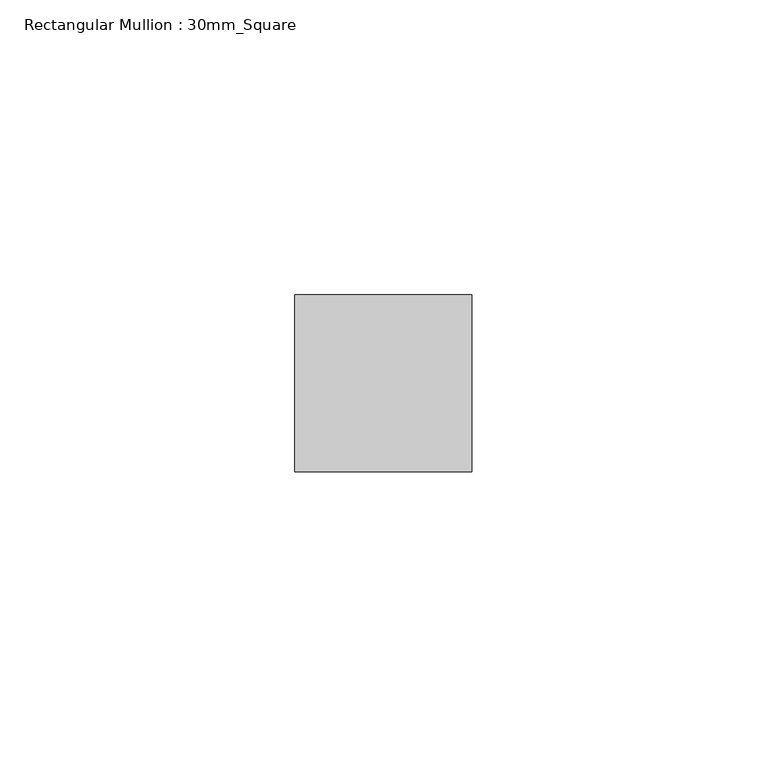
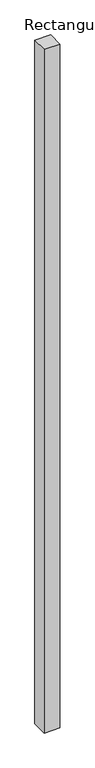
"""IFC4 building model written with IfcOpenShell, lengths in millimetres: member geometry, Rectangular Mullion : 30mm_Square."""

from ifc_helpers import new_model, si_unit, frame, origin, place, context, project, spatial, polyline, outline, extrude, source, transform, mapped, element, save


def rectangular_mullion_30mm_square_48e0410f(model_context):
    return source(origin(), model_context, "Body", "SweptSolid", [
        extrude(outline(polyline([(0.0, 15.0), (0.0, -15.0), (-30.0, -15.0), (-30.0, 15.0), (0.0, 15.0)])), frame((0.0, 0.0, -1366.1782299), z_axis=(0.0, 0.0, 1.0), x_axis=(1.0, 0.0, 0.0)), (0.0, 0.0, 1.0), 1366.1782299),
    ])


if __name__ == "__main__":
    model = new_model("IFC4")
    model_context = context("Model", 3, world=origin())
    ifc_project = project(units=[si_unit("LENGTHUNIT", "METRE", prefix="MILLI")], contexts=[model_context])
    site = spatial("IfcSite", under=ifc_project)
    building = spatial("IfcBuilding", under=site)
    placement = place(None, origin())
    rectangular_mullion_30mm_square_shape = rectangular_mullion_30mm_square_48e0410f(model_context)
    element("IfcMember", 1, ObjectType="Rectangular Mullion : 30mm_Square", at=placement, inside=building, context=model_context, shape_type="MappedRepresentation", body=[
        mapped(rectangular_mullion_30mm_square_shape, transform((0.0, 0.0, 0.0), x_axis=(1.0, 0.0, 0.0), y_axis=(0.0, 1.0, 0.0), z_axis=(0.0, 0.0, 1.0))),
    ])
    save(model, "model.ifc")

# Revit data of these elements
# Type "Rectangular Mullion : 30mm_Square"
#   Keynote = "H11"
#   built-in parameter 1007304 = 0.0984252 (stored number, unit not read)
#   built-in parameter 1007301 = 0.0492126 (stored number, unit not read)
#   built-in parameter 1007300 = 0.0492126 (stored number, unit not read)
# Element 1 (IfcMember, "Rectangular Mullion : 30mm_Square")
#   Materials on its faces: "Aluminium"
# Materials
#   "Aluminium": class "Metal", colour RGB 247 247 247, transparency 0, Description = "Aluminium 6061", Cost = 0
